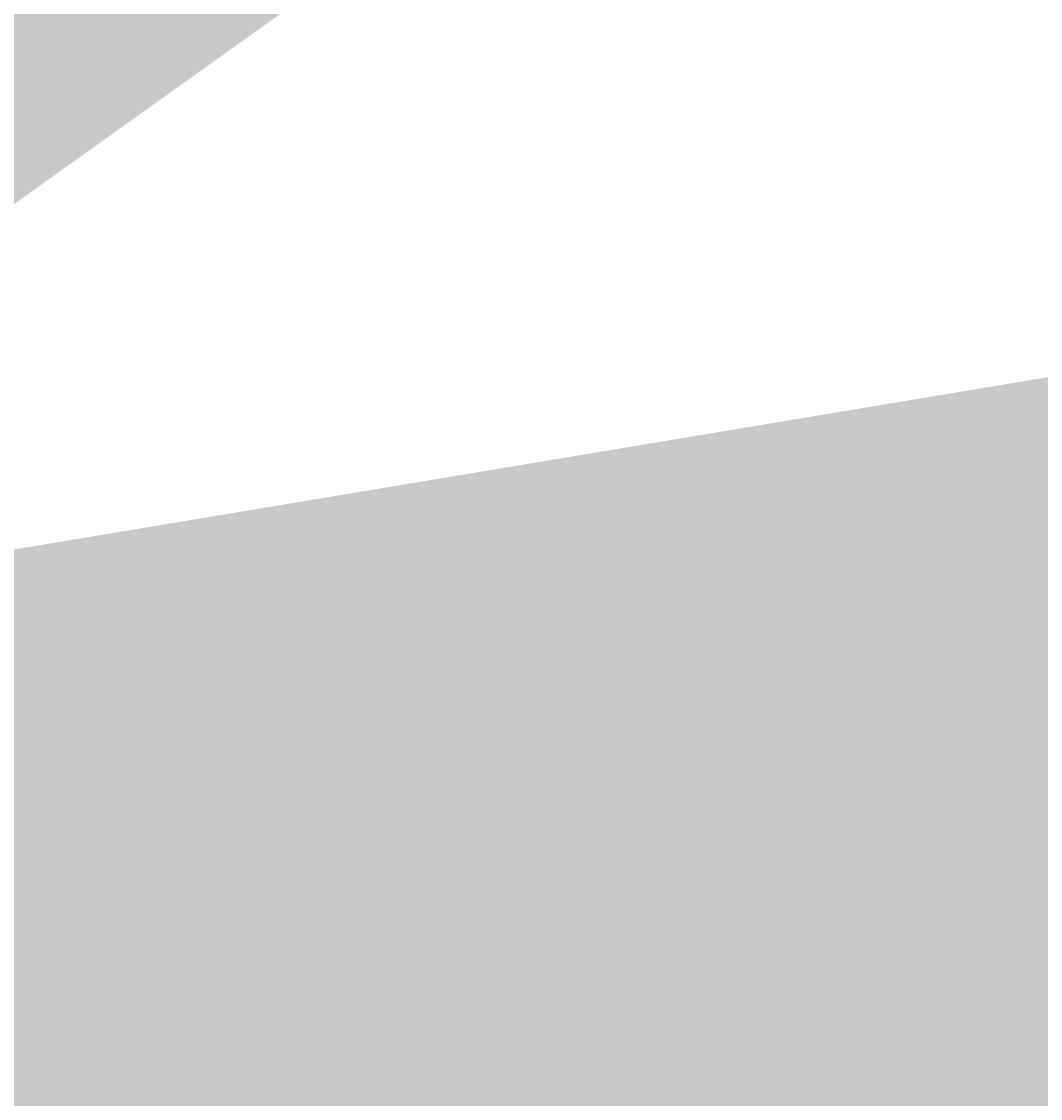
# Model space of a CAD drawing. Units: millimetres. Extents: x -22994 to 29398, y -19990 to 20176.
# Tile 129 of 135: x 1004 to 2052, y -212 to 895. Entities that reach past the tile are written whole.
import ezdxf

# ---------------------------------------------------------------- set-up
doc = ezdxf.new("R2010")
doc.units = ezdxf.units.MM
doc.header["$MEASUREMENT"] = 0
doc.layers.add('M-DIMS', color=2, linetype='Continuous', lineweight=18)
doc.styles.get("Standard").update_dxf_attribs({"font": 'arial.ttf'})
doc.dimstyles.get("Standard").update_dxf_attribs({"dimtxt": 0.18, "dimasz": 10000, "dimexe": 0.18, "dimexo": 0.0625, "dimgap": 0.09, "dimtad": 0, "dimtih": 1, "dimtoh": 1, "dimdec": 0, "dimzin": 0, "dimdsep": 46, "dimtxsty": 'Standard', "dimcen": 0.09, "dimadec": 0, "dimazin": 0, "dimtfac": 1, "dimtdec": 0, "dimtofl": 0, "dimtmove": 0, "dimatfit": 3, "dimfxl": 1, "dimtolj": 1, "dimtzin": 0, "dimlwd": 30, "dimarcsym": 0})

# ---------------------------------------------------------------- blocks, each defined once
blk = doc.blocks.new('*D2')
at = {"layer": 'Defpoints', "color": 0, "transparency": 16777216}
for p in [(6.7, 10.3), (290.9, 10.3), (290.9, -5.1)]:
    blk.add_point(p, dxfattribs=at)
at = {"layer": 'M-DIMS', "color": 0, "lineweight": -2, "transparency": 16777216}
for p, q in [((6.7, 10.2), (6.7, -5.3)), ((290.9, 10.2), (290.9, -5.3))]:
    blk.add_line(p, q, dxfattribs=at)
at = {"layer": 'M-DIMS', "color": 0, "lineweight": 30, "transparency": 16777216}
for p, q in [((-9993.3, -5.1), (-19993.3, -5.1)), ((10290.9, -5.1), (20290.9, -5.1))]:
    blk.add_line(p, q, dxfattribs=at)
at = {"layer": 'M-DIMS', "color": 0, "transparency": 16777216}
for points in [[(-9993.3, 1661.6), (-9993.3, -1671.7), (6.7, -5.1)], [(10290.9, 1661.6), (10290.9, -1671.7), (290.9, -5.1)]]:
    blk.add_solid(points, dxfattribs=at)
at = {"layer": 'M-DIMS', "color": 0, "transparency": 16777216, "insert": (148.8, -5.1), "char_height": 0.18, "attachment_point": 5}
blk.add_mtext('\\A1;284.2', dxfattribs=at)
blk = doc.blocks.new('*D3')
at = {"layer": 'Defpoints', "color": 0, "transparency": 16777216}
for p in [(110.3, 204.2), (110.3, 176.4), (95.8, 128)]:
    blk.add_point(p, dxfattribs=at)
at = {"layer": 'M-DIMS', "color": 0, "lineweight": 30, "transparency": 16777216}
for p, q in [((-9904.2, 204.2), (-19904.2, 204.2)), ((10110.3, 204.2), (20110.3, 204.2))]:
    blk.add_line(p, q, dxfattribs=at)
at = {"layer": 'M-DIMS', "color": 0, "lineweight": -2, "transparency": 16777216}
for p, q in [((95.8, 128), (95.8, 204.3)), ((110.3, 176.4), (110.3, 204.3))]:
    blk.add_line(p, q, dxfattribs=at)
at = {"layer": 'M-DIMS', "color": 0, "transparency": 16777216}
for points in [[(-9904.2, 1870.8), (-9904.2, -1462.5), (95.8, 204.2)], [(10110.3, 1870.8), (10110.3, -1462.5), (110.3, 204.2)]]:
    blk.add_solid(points, dxfattribs=at)
at = {"layer": 'M-DIMS', "color": 0, "transparency": 16777216, "insert": (103, 204.2), "char_height": 0.18, "attachment_point": 5}
blk.add_mtext('\\A1;14.432', dxfattribs=at)
blk = doc.blocks.new('*D4')
at = {"layer": 'Defpoints', "color": 0, "transparency": 16777216}
for p in [(116.3, 204.2), (110.3, 176.4), (116.3, 176.4)]:
    blk.add_point(p, dxfattribs=at)
at = {"layer": 'M-DIMS', "color": 0, "lineweight": 30, "transparency": 16777216}
for p, q in [((-9889.7, 204.2), (-19889.7, 204.2)), ((10116.3, 204.2), (20116.3, 204.2))]:
    blk.add_line(p, q, dxfattribs=at)
at = {"layer": 'M-DIMS', "color": 0, "lineweight": -2, "transparency": 16777216}
for p, q in [((110.3, 176.4), (110.3, 204.3)), ((116.3, 176.4), (116.3, 204.3))]:
    blk.add_line(p, q, dxfattribs=at)
at = {"layer": 'M-DIMS', "color": 0, "transparency": 16777216}
for points in [[(-9889.7, 1870.8), (-9889.7, -1462.5), (110.3, 204.2)], [(10116.3, 1870.8), (10116.3, -1462.5), (116.3, 204.2)]]:
    blk.add_solid(points, dxfattribs=at)
at = {"layer": 'M-DIMS', "color": 0, "transparency": 16777216, "insert": (113.3, 204.2), "char_height": 0.18, "attachment_point": 5}
blk.add_mtext('\\A1;6', dxfattribs=at)
blk = doc.blocks.new('*D5')
at = {"layer": 'Defpoints', "color": 0, "transparency": 16777216}
for p in [(181.3, 204.2), (116.3, 176.4), (181.3, 176.4)]:
    blk.add_point(p, dxfattribs=at)
at = {"layer": 'M-DIMS', "color": 0, "lineweight": 30, "transparency": 16777216}
for p, q in [((-9883.7, 204.2), (-19883.7, 204.2)), ((10181.3, 204.2), (20181.3, 204.2))]:
    blk.add_line(p, q, dxfattribs=at)
at = {"layer": 'M-DIMS', "color": 0, "lineweight": -2, "transparency": 16777216}
for p, q in [((116.3, 176.4), (116.3, 204.3)), ((181.3, 176.4), (181.3, 204.3))]:
    blk.add_line(p, q, dxfattribs=at)
at = {"layer": 'M-DIMS', "color": 0, "transparency": 16777216}
for points in [[(-9883.7, 1870.8), (-9883.7, -1462.5), (116.3, 204.2)], [(10181.3, 1870.8), (10181.3, -1462.5), (181.3, 204.2)]]:
    blk.add_solid(points, dxfattribs=at)
at = {"layer": 'M-DIMS', "color": 0, "transparency": 16777216, "insert": (148.8, 204.2), "char_height": 0.18, "attachment_point": 5}
blk.add_mtext('\\A1;65', dxfattribs=at)
blk = doc.blocks.new('*D6')
at = {"layer": 'Defpoints', "color": 0, "transparency": 16777216}
for p in [(187.3, 204.2), (181.3, 176.4), (187.3, 176.4)]:
    blk.add_point(p, dxfattribs=at)
at = {"layer": 'M-DIMS', "color": 0, "lineweight": 30, "transparency": 16777216}
for p, q in [((-9818.7, 204.2), (-19818.7, 204.2)), ((10187.3, 204.2), (20187.3, 204.2))]:
    blk.add_line(p, q, dxfattribs=at)
at = {"layer": 'M-DIMS', "color": 0, "lineweight": -2, "transparency": 16777216}
for p, q in [((181.3, 176.4), (181.3, 204.3)), ((187.3, 176.4), (187.3, 204.3))]:
    blk.add_line(p, q, dxfattribs=at)
at = {"layer": 'M-DIMS', "color": 0, "transparency": 16777216}
for points in [[(-9818.7, 1870.8), (-9818.7, -1462.5), (181.3, 204.2)], [(10187.3, 1870.8), (10187.3, -1462.5), (187.3, 204.2)]]:
    blk.add_solid(points, dxfattribs=at)
at = {"layer": 'M-DIMS', "color": 0, "transparency": 16777216, "insert": (184.3, 204.2), "char_height": 0.18, "attachment_point": 5}
blk.add_mtext('\\A1;6', dxfattribs=at)
blk = doc.blocks.new('*D7')
at = {"layer": 'Defpoints', "color": 0, "transparency": 16777216}
for p in [(201.7, 204.2), (187.3, 176.4), (201.7, 128)]:
    blk.add_point(p, dxfattribs=at)
at = {"layer": 'M-DIMS', "color": 0, "lineweight": 30, "transparency": 16777216}
for p, q in [((-9812.7, 204.2), (-19812.7, 204.2)), ((10201.7, 204.2), (20201.7, 204.2))]:
    blk.add_line(p, q, dxfattribs=at)
at = {"layer": 'M-DIMS', "color": 0, "lineweight": -2, "transparency": 16777216}
for p, q in [((187.3, 176.4), (187.3, 204.3)), ((201.7, 128), (201.7, 204.3))]:
    blk.add_line(p, q, dxfattribs=at)
at = {"layer": 'M-DIMS', "color": 0, "transparency": 16777216}
for points in [[(-9812.7, 1870.8), (-9812.7, -1462.5), (187.3, 204.2)], [(10201.7, 1870.8), (10201.7, -1462.5), (201.7, 204.2)]]:
    blk.add_solid(points, dxfattribs=at)
at = {"layer": 'M-DIMS', "color": 0, "transparency": 16777216, "insert": (194.5, 204.2), "char_height": 0.18, "attachment_point": 5}
blk.add_mtext('\\A1;14.432', dxfattribs=at)
blk = doc.blocks.new('*D8')
at = {"layer": 'Defpoints', "color": 0, "transparency": 16777216}
for p in [(227.6, 204.2), (227.6, 146.7), (201.7, 128)]:
    blk.add_point(p, dxfattribs=at)
at = {"layer": 'M-DIMS', "color": 0, "lineweight": 30, "transparency": 16777216}
for p, q in [((-9798.3, 204.2), (-19798.3, 204.2)), ((10227.6, 204.2), (20227.6, 204.2))]:
    blk.add_line(p, q, dxfattribs=at)
at = {"layer": 'M-DIMS', "color": 0, "lineweight": -2, "transparency": 16777216}
for p, q in [((201.7, 128), (201.7, 204.3)), ((227.6, 146.8), (227.6, 204.3))]:
    blk.add_line(p, q, dxfattribs=at)
at = {"layer": 'M-DIMS', "color": 0, "transparency": 16777216}
for points in [[(-9798.3, 1870.8), (-9798.3, -1462.5), (201.7, 204.2)], [(10227.6, 1870.8), (10227.6, -1462.5), (227.6, 204.2)]]:
    blk.add_solid(points, dxfattribs=at)
at = {"layer": 'M-DIMS', "color": 0, "transparency": 16777216, "insert": (214.7, 204.2), "char_height": 0.18, "attachment_point": 5}
blk.add_mtext('\\A1;25.95', dxfattribs=at)
blk = doc.blocks.new('*D9')
at = {"layer": 'Defpoints', "color": 0, "transparency": 16777216}
for p in [(187.3, 176.4), (306.2, 176.4), (290.9, 10.3)]:
    blk.add_point(p, dxfattribs=at)
at = {"layer": 'M-DIMS', "color": 0, "lineweight": 30, "transparency": 16777216}
for p, q in [((306.2, 10176.4), (306.2, 20176.4)), ((306.2, -9989.7), (306.2, -19989.7))]:
    blk.add_line(p, q, dxfattribs=at)
at = {"layer": 'M-DIMS', "color": 0, "lineweight": -2, "transparency": 16777216}
for p, q in [((187.3, 176.4), (306.4, 176.4)), ((290.9, 10.3), (306.4, 10.3))]:
    blk.add_line(p, q, dxfattribs=at)
at = {"layer": 'M-DIMS', "color": 0, "transparency": 16777216}
for points in [[(-1360.5, 10176.4), (1972.9, 10176.4), (306.2, 176.4)], [(-1360.5, -9989.7), (1972.9, -9989.7), (306.2, 10.3)]]:
    blk.add_solid(points, dxfattribs=at)
at = {"layer": 'M-DIMS', "color": 0, "transparency": 16777216, "insert": (306.2, 93.3), "char_height": 0.18, "attachment_point": 5}
blk.add_mtext('\\A1;166.1', dxfattribs=at)
blk = doc.blocks.new('*D10')
at = {"layer": 'Defpoints', "color": 0, "transparency": 16777216}
for p in [(125.6, 136.1), (133.3, 136.1), (133.3, -5.1)]:
    blk.add_point(p, dxfattribs=at)
at = {"layer": 'M-DIMS', "color": 0, "lineweight": -2, "transparency": 16777216}
for p, q in [((125.6, 136), (125.6, -5.3)), ((133.3, 136), (133.3, -5.3))]:
    blk.add_line(p, q, dxfattribs=at)
at = {"layer": 'M-DIMS', "color": 0, "lineweight": 30, "transparency": 16777216}
for p, q in [((-9874.4, -5.1), (-19874.4, -5.1)), ((10133.3, -5.1), (20133.3, -5.1))]:
    blk.add_line(p, q, dxfattribs=at)
at = {"layer": 'M-DIMS', "color": 0, "transparency": 16777216}
for points in [[(-9874.4, 1661.6), (-9874.4, -1671.7), (125.6, -5.1)], [(10133.3, 1661.6), (10133.3, -1671.7), (133.3, -5.1)]]:
    blk.add_solid(points, dxfattribs=at)
at = {"layer": 'M-DIMS', "color": 0, "transparency": 16777216, "insert": (129.5, -5.1), "char_height": 0.18, "attachment_point": 5}
blk.add_mtext('\\A1;7.696', dxfattribs=at)
blk = doc.blocks.new('*D11')
at = {"layer": 'Defpoints', "color": 0, "transparency": 16777216}
for p in [(133.3, 136.1), (135.6, 136.1), (135.6, -5.1)]:
    blk.add_point(p, dxfattribs=at)
at = {"layer": 'M-DIMS', "color": 0, "lineweight": -2, "transparency": 16777216}
for p, q in [((133.3, 136), (133.3, -5.3)), ((135.6, 136), (135.6, -5.3))]:
    blk.add_line(p, q, dxfattribs=at)
at = {"layer": 'M-DIMS', "color": 0, "lineweight": 30, "transparency": 16777216}
for p, q in [((-9866.7, -5.1), (-19866.7, -5.1)), ((10135.6, -5.1), (20135.6, -5.1))]:
    blk.add_line(p, q, dxfattribs=at)
at = {"layer": 'M-DIMS', "color": 0, "transparency": 16777216}
for points in [[(-9866.7, 1661.6), (-9866.7, -1671.7), (133.3, -5.1)], [(10135.6, 1661.6), (10135.6, -1671.7), (135.6, -5.1)]]:
    blk.add_solid(points, dxfattribs=at)
at = {"layer": 'M-DIMS', "color": 0, "transparency": 16777216, "insert": (134.5, -5.1), "char_height": 0.18, "attachment_point": 5}
blk.add_mtext('\\A1;2.304', dxfattribs=at)
blk = doc.blocks.new('*D12')
at = {"layer": 'Defpoints', "color": 0, "transparency": 16777216}
for p in [(135.6, 136.1), (145.6, 136.1), (145.6, -5.1)]:
    blk.add_point(p, dxfattribs=at)
at = {"layer": 'M-DIMS', "color": 0, "lineweight": -2, "transparency": 16777216}
for p, q in [((135.6, 136), (135.6, -5.3)), ((145.6, 136), (145.6, -5.3))]:
    blk.add_line(p, q, dxfattribs=at)
at = {"layer": 'M-DIMS', "color": 0, "lineweight": 30, "transparency": 16777216}
for p, q in [((-9864.4, -5.1), (-19864.4, -5.1)), ((10145.6, -5.1), (20145.6, -5.1))]:
    blk.add_line(p, q, dxfattribs=at)
at = {"layer": 'M-DIMS', "color": 0, "transparency": 16777216}
for points in [[(-9864.4, 1661.6), (-9864.4, -1671.7), (135.6, -5.1)], [(10145.6, 1661.6), (10145.6, -1671.7), (145.6, -5.1)]]:
    blk.add_solid(points, dxfattribs=at)
at = {"layer": 'M-DIMS', "color": 0, "transparency": 16777216, "insert": (140.6, -5.1), "char_height": 0.18, "attachment_point": 5}
blk.add_mtext('\\A1;10', dxfattribs=at)
blk = doc.blocks.new('*D13')
at = {"layer": 'Defpoints', "color": 0, "transparency": 16777216}
for p in [(145.6, 136.1), (155.6, 136.1), (155.6, -5.1)]:
    blk.add_point(p, dxfattribs=at)
at = {"layer": 'M-DIMS', "color": 0, "lineweight": -2, "transparency": 16777216}
for p, q in [((145.6, 136), (145.6, -5.3)), ((155.6, 136), (155.6, -5.3))]:
    blk.add_line(p, q, dxfattribs=at)
at = {"layer": 'M-DIMS', "color": 0, "lineweight": 30, "transparency": 16777216}
for p, q in [((-9854.4, -5.1), (-19854.4, -5.1)), ((10155.6, -5.1), (20155.6, -5.1))]:
    blk.add_line(p, q, dxfattribs=at)
at = {"layer": 'M-DIMS', "color": 0, "transparency": 16777216}
for points in [[(-9854.4, 1661.6), (-9854.4, -1671.7), (145.6, -5.1)], [(10155.6, 1661.6), (10155.6, -1671.7), (155.6, -5.1)]]:
    blk.add_solid(points, dxfattribs=at)
at = {"layer": 'M-DIMS', "color": 0, "transparency": 16777216, "insert": (150.6, -5.1), "char_height": 0.18, "attachment_point": 5}
blk.add_mtext('\\A1;10', dxfattribs=at)
blk = doc.blocks.new('*D14')
at = {"layer": 'Defpoints', "color": 0, "transparency": 16777216}
for p in [(155.6, 136.1), (165.6, 136.1), (165.6, -5.1)]:
    blk.add_point(p, dxfattribs=at)
at = {"layer": 'M-DIMS', "color": 0, "lineweight": -2, "transparency": 16777216}
for p, q in [((155.6, 136), (155.6, -5.3)), ((165.6, 136), (165.6, -5.3))]:
    blk.add_line(p, q, dxfattribs=at)
at = {"layer": 'M-DIMS', "color": 0, "lineweight": 30, "transparency": 16777216}
for p, q in [((-9844.4, -5.1), (-19844.4, -5.1)), ((10165.6, -5.1), (20165.6, -5.1))]:
    blk.add_line(p, q, dxfattribs=at)
at = {"layer": 'M-DIMS', "color": 0, "transparency": 16777216}
for points in [[(-9844.4, 1661.6), (-9844.4, -1671.7), (155.6, -5.1)], [(10165.6, 1661.6), (10165.6, -1671.7), (165.6, -5.1)]]:
    blk.add_solid(points, dxfattribs=at)
at = {"layer": 'M-DIMS', "color": 0, "transparency": 16777216, "insert": (160.6, -5.1), "char_height": 0.18, "attachment_point": 5}
blk.add_mtext('\\A1;10', dxfattribs=at)
blk = doc.blocks.new('*D15')
at = {"layer": 'Defpoints', "color": 0, "transparency": 16777216}
for p in [(173.3, 154.8), (173.3, 136.1), (306.2, 136.1)]:
    blk.add_point(p, dxfattribs=at)
at = {"layer": 'M-DIMS', "color": 0, "lineweight": 30, "transparency": 16777216}
for p, q in [((306.2, 10154.8), (306.2, 20154.8)), ((306.2, -9863.9), (306.2, -19863.9))]:
    blk.add_line(p, q, dxfattribs=at)
at = {"layer": 'M-DIMS', "color": 0, "lineweight": -2, "transparency": 16777216}
for p, q in [((173.4, 154.8), (306.4, 154.8)), ((173.4, 136.1), (306.4, 136.1))]:
    blk.add_line(p, q, dxfattribs=at)
at = {"layer": 'M-DIMS', "color": 0, "transparency": 16777216}
for points in [[(-1360.5, 10154.8), (1972.9, 10154.8), (306.2, 154.8)], [(-1360.5, -9863.9), (1972.9, -9863.9), (306.2, 136.1)]]:
    blk.add_solid(points, dxfattribs=at)
at = {"layer": 'M-DIMS', "color": 0, "transparency": 16777216, "insert": (306.2, 145.4), "char_height": 0.18, "attachment_point": 5}
blk.add_mtext('\\A1;18.717', dxfattribs=at)
blk = doc.blocks.new('*D16')
at = {"layer": 'Defpoints', "color": 0, "transparency": 16777216}
for p in [(120.2, 204.2), (110.5, 48), (120.2, 48)]:
    blk.add_point(p, dxfattribs=at)
at = {"layer": 'M-DIMS', "color": 0, "lineweight": 30, "transparency": 16777216}
for p, q in [((-9889.5, 204.2), (-19889.5, 204.2)), ((10120.2, 204.2), (20120.2, 204.2))]:
    blk.add_line(p, q, dxfattribs=at)
at = {"layer": 'M-DIMS', "color": 0, "lineweight": -2, "transparency": 16777216}
for p, q in [((110.5, 48.1), (110.5, 204.3)), ((120.2, 48.1), (120.2, 204.3))]:
    blk.add_line(p, q, dxfattribs=at)
at = {"layer": 'M-DIMS', "color": 0, "transparency": 16777216}
for points in [[(-9889.5, 1870.8), (-9889.5, -1462.5), (110.5, 204.2)], [(10120.2, 1870.8), (10120.2, -1462.5), (120.2, 204.2)]]:
    blk.add_solid(points, dxfattribs=at)
at = {"layer": 'M-DIMS', "color": 0, "transparency": 16777216, "insert": (115.3, 204.2), "char_height": 0.18, "attachment_point": 5}
blk.add_mtext('\\A1;9.704', dxfattribs=at)
blk = doc.blocks.new('*D17')
at = {"layer": 'Defpoints', "color": 0, "transparency": 16777216}
for p in [(126.2, 204.2), (120.2, 48), (126.2, 48)]:
    blk.add_point(p, dxfattribs=at)
at = {"layer": 'M-DIMS', "color": 0, "lineweight": 30, "transparency": 16777216}
for p, q in [((-9879.8, 204.2), (-19879.8, 204.2)), ((10126.2, 204.2), (20126.2, 204.2))]:
    blk.add_line(p, q, dxfattribs=at)
at = {"layer": 'M-DIMS', "color": 0, "lineweight": -2, "transparency": 16777216}
for p, q in [((120.2, 48.1), (120.2, 204.3)), ((126.2, 48.1), (126.2, 204.3))]:
    blk.add_line(p, q, dxfattribs=at)
at = {"layer": 'M-DIMS', "color": 0, "transparency": 16777216}
for points in [[(-9879.8, 1870.8), (-9879.8, -1462.5), (120.2, 204.2)], [(10126.2, 1870.8), (10126.2, -1462.5), (126.2, 204.2)]]:
    blk.add_solid(points, dxfattribs=at)
at = {"layer": 'M-DIMS', "color": 0, "transparency": 16777216, "insert": (123.2, 204.2), "char_height": 0.18, "attachment_point": 5}
blk.add_mtext('\\A1;6', dxfattribs=at)
blk = doc.blocks.new('*D18')
at = {"layer": 'Defpoints', "color": 0, "transparency": 16777216}
for p in [(132.2, 204.2), (126.2, 48), (132.2, 48)]:
    blk.add_point(p, dxfattribs=at)
at = {"layer": 'M-DIMS', "color": 0, "lineweight": 30, "transparency": 16777216}
for p, q in [((-9873.8, 204.2), (-19873.8, 204.2)), ((10132.2, 204.2), (20132.2, 204.2))]:
    blk.add_line(p, q, dxfattribs=at)
at = {"layer": 'M-DIMS', "color": 0, "lineweight": -2, "transparency": 16777216}
for p, q in [((126.2, 48.1), (126.2, 204.3)), ((132.2, 48.1), (132.2, 204.3))]:
    blk.add_line(p, q, dxfattribs=at)
at = {"layer": 'M-DIMS', "color": 0, "transparency": 16777216}
for points in [[(-9873.8, 1870.8), (-9873.8, -1462.5), (126.2, 204.2)], [(10132.2, 1870.8), (10132.2, -1462.5), (132.2, 204.2)]]:
    blk.add_solid(points, dxfattribs=at)
at = {"layer": 'M-DIMS', "color": 0, "transparency": 16777216, "insert": (129.2, 204.2), "char_height": 0.18, "attachment_point": 5}
blk.add_mtext('\\A1;6', dxfattribs=at)
blk = doc.blocks.new('*D19')
at = {"layer": 'Defpoints', "color": 0, "transparency": 16777216}
for p in [(138.2, 204.2), (132.2, 48), (138.2, 48)]:
    blk.add_point(p, dxfattribs=at)
at = {"layer": 'M-DIMS', "color": 0, "lineweight": 30, "transparency": 16777216}
for p, q in [((-9867.8, 204.2), (-19867.8, 204.2)), ((10138.2, 204.2), (20138.2, 204.2))]:
    blk.add_line(p, q, dxfattribs=at)
at = {"layer": 'M-DIMS', "color": 0, "lineweight": -2, "transparency": 16777216}
for p, q in [((132.2, 48.1), (132.2, 204.3)), ((138.2, 48.1), (138.2, 204.3))]:
    blk.add_line(p, q, dxfattribs=at)
at = {"layer": 'M-DIMS', "color": 0, "transparency": 16777216}
for points in [[(-9867.8, 1870.8), (-9867.8, -1462.5), (132.2, 204.2)], [(10138.2, 1870.8), (10138.2, -1462.5), (138.2, 204.2)]]:
    blk.add_solid(points, dxfattribs=at)
at = {"layer": 'M-DIMS', "color": 0, "transparency": 16777216, "insert": (135.2, 204.2), "char_height": 0.18, "attachment_point": 5}
blk.add_mtext('\\A1;6', dxfattribs=at)
blk = doc.blocks.new('*D20')
at = {"layer": 'Defpoints', "color": 0, "transparency": 16777216}
for p in [(144.2, 204.2), (138.2, 48), (144.2, 48)]:
    blk.add_point(p, dxfattribs=at)
at = {"layer": 'M-DIMS', "color": 0, "lineweight": 30, "transparency": 16777216}
for p, q in [((-9861.8, 204.2), (-19861.8, 204.2)), ((10144.2, 204.2), (20144.2, 204.2))]:
    blk.add_line(p, q, dxfattribs=at)
at = {"layer": 'M-DIMS', "color": 0, "lineweight": -2, "transparency": 16777216}
for p, q in [((138.2, 48.1), (138.2, 204.3)), ((144.2, 48.1), (144.2, 204.3))]:
    blk.add_line(p, q, dxfattribs=at)
at = {"layer": 'M-DIMS', "color": 0, "transparency": 16777216}
for points in [[(-9861.8, 1870.8), (-9861.8, -1462.5), (138.2, 204.2)], [(10144.2, 1870.8), (10144.2, -1462.5), (144.2, 204.2)]]:
    blk.add_solid(points, dxfattribs=at)
at = {"layer": 'M-DIMS', "color": 0, "transparency": 16777216, "insert": (141.2, 204.2), "char_height": 0.18, "attachment_point": 5}
blk.add_mtext('\\A1;6', dxfattribs=at)
blk = doc.blocks.new('*D21')
at = {"layer": 'Defpoints', "color": 0, "transparency": 16777216}
for p in [(149.1, 204.2), (144.2, 48), (149.1, 48)]:
    blk.add_point(p, dxfattribs=at)
at = {"layer": 'M-DIMS', "color": 0, "lineweight": 30, "transparency": 16777216}
for p, q in [((-9855.8, 204.2), (-19855.8, 204.2)), ((10149.1, 204.2), (20149.1, 204.2))]:
    blk.add_line(p, q, dxfattribs=at)
at = {"layer": 'M-DIMS', "color": 0, "lineweight": -2, "transparency": 16777216}
for p, q in [((144.2, 48.1), (144.2, 204.3)), ((149.1, 48.1), (149.1, 204.3))]:
    blk.add_line(p, q, dxfattribs=at)
at = {"layer": 'M-DIMS', "color": 0, "transparency": 16777216}
for points in [[(-9855.8, 1870.8), (-9855.8, -1462.5), (144.2, 204.2)], [(10149.1, 1870.8), (10149.1, -1462.5), (149.1, 204.2)]]:
    blk.add_solid(points, dxfattribs=at)
at = {"layer": 'M-DIMS', "color": 0, "transparency": 16777216, "insert": (146.6, 204.2), "char_height": 0.18, "attachment_point": 5}
blk.add_mtext('\\A1;4.945', dxfattribs=at)
blk = doc.blocks.new('*D22')
at = {"layer": 'Defpoints', "color": 0, "transparency": 16777216}
for p in [(149.1, 31), (155.1, 31), (155.1, -5.1)]:
    blk.add_point(p, dxfattribs=at)
at = {"layer": 'M-DIMS', "color": 0, "lineweight": -2, "transparency": 16777216}
for p, q in [((149.1, 30.9), (149.1, -5.3)), ((155.1, 30.9), (155.1, -5.3))]:
    blk.add_line(p, q, dxfattribs=at)
at = {"layer": 'M-DIMS', "color": 0, "lineweight": 30, "transparency": 16777216}
for p, q in [((-9850.9, -5.1), (-19850.9, -5.1)), ((10155.1, -5.1), (20155.1, -5.1))]:
    blk.add_line(p, q, dxfattribs=at)
at = {"layer": 'M-DIMS', "color": 0, "transparency": 16777216}
for points in [[(-9850.9, 1661.6), (-9850.9, -1671.7), (149.1, -5.1)], [(10155.1, 1661.6), (10155.1, -1671.7), (155.1, -5.1)]]:
    blk.add_solid(points, dxfattribs=at)
at = {"layer": 'M-DIMS', "color": 0, "transparency": 16777216, "insert": (152.1, -5.1), "char_height": 0.18, "attachment_point": 5}
blk.add_mtext('\\A1;6', dxfattribs=at)
blk = doc.blocks.new('*D23')
at = {"layer": 'Defpoints', "color": 0, "transparency": 16777216}
for p in [(155.1, 31), (161.1, 31), (161.1, -5.1)]:
    blk.add_point(p, dxfattribs=at)
at = {"layer": 'M-DIMS', "color": 0, "lineweight": -2, "transparency": 16777216}
for p, q in [((155.1, 30.9), (155.1, -5.3)), ((161.1, 30.9), (161.1, -5.3))]:
    blk.add_line(p, q, dxfattribs=at)
at = {"layer": 'M-DIMS', "color": 0, "lineweight": 30, "transparency": 16777216}
for p, q in [((-9844.9, -5.1), (-19844.9, -5.1)), ((10161.1, -5.1), (20161.1, -5.1))]:
    blk.add_line(p, q, dxfattribs=at)
at = {"layer": 'M-DIMS', "color": 0, "transparency": 16777216}
for points in [[(-9844.9, 1661.6), (-9844.9, -1671.7), (155.1, -5.1)], [(10161.1, 1661.6), (10161.1, -1671.7), (161.1, -5.1)]]:
    blk.add_solid(points, dxfattribs=at)
at = {"layer": 'M-DIMS', "color": 0, "transparency": 16777216, "insert": (158.1, -5.1), "char_height": 0.18, "attachment_point": 5}
blk.add_mtext('\\A1;6', dxfattribs=at)
blk = doc.blocks.new('*D24')
at = {"layer": 'Defpoints', "color": 0, "transparency": 16777216}
for p in [(161.1, 31), (166.4, 31), (166.4, -5.1)]:
    blk.add_point(p, dxfattribs=at)
at = {"layer": 'M-DIMS', "color": 0, "lineweight": -2, "transparency": 16777216}
for p, q in [((161.1, 30.9), (161.1, -5.3)), ((166.4, 30.9), (166.4, -5.3))]:
    blk.add_line(p, q, dxfattribs=at)
at = {"layer": 'M-DIMS', "color": 0, "lineweight": 30, "transparency": 16777216}
for p, q in [((-9838.9, -5.1), (-19838.9, -5.1)), ((10166.4, -5.1), (20166.4, -5.1))]:
    blk.add_line(p, q, dxfattribs=at)
at = {"layer": 'M-DIMS', "color": 0, "transparency": 16777216}
for points in [[(-9838.9, 1661.6), (-9838.9, -1671.7), (161.1, -5.1)], [(10166.4, 1661.6), (10166.4, -1671.7), (166.4, -5.1)]]:
    blk.add_solid(points, dxfattribs=at)
at = {"layer": 'M-DIMS', "color": 0, "transparency": 16777216, "insert": (163.8, -5.1), "char_height": 0.18, "attachment_point": 5}
blk.add_mtext('\\A1;5.323', dxfattribs=at)
blk = doc.blocks.new('*D25')
at = {"layer": 'Defpoints', "color": 0, "transparency": 16777216}
for p in [(166.4, 31), (172.4, 31), (172.4, -5.1)]:
    blk.add_point(p, dxfattribs=at)
at = {"layer": 'M-DIMS', "color": 0, "lineweight": -2, "transparency": 16777216}
for p, q in [((166.4, 30.9), (166.4, -5.3)), ((172.4, 30.9), (172.4, -5.3))]:
    blk.add_line(p, q, dxfattribs=at)
at = {"layer": 'M-DIMS', "color": 0, "lineweight": 30, "transparency": 16777216}
for p, q in [((-9833.6, -5.1), (-19833.6, -5.1)), ((10172.4, -5.1), (20172.4, -5.1))]:
    blk.add_line(p, q, dxfattribs=at)
at = {"layer": 'M-DIMS', "color": 0, "transparency": 16777216}
for points in [[(-9833.6, 1661.6), (-9833.6, -1671.7), (166.4, -5.1)], [(10172.4, 1661.6), (10172.4, -1671.7), (172.4, -5.1)]]:
    blk.add_solid(points, dxfattribs=at)
at = {"layer": 'M-DIMS', "color": 0, "transparency": 16777216, "insert": (169.4, -5.1), "char_height": 0.18, "attachment_point": 5}
blk.add_mtext('\\A1;6', dxfattribs=at)
blk = doc.blocks.new('*D26')
at = {"layer": 'Defpoints', "color": 0, "transparency": 16777216}
for p in [(172.4, 31), (178.4, 31), (178.4, -5.1)]:
    blk.add_point(p, dxfattribs=at)
at = {"layer": 'M-DIMS', "color": 0, "lineweight": -2, "transparency": 16777216}
for p, q in [((172.4, 30.9), (172.4, -5.3)), ((178.4, 30.9), (178.4, -5.3))]:
    blk.add_line(p, q, dxfattribs=at)
at = {"layer": 'M-DIMS', "color": 0, "lineweight": 30, "transparency": 16777216}
for p, q in [((-9827.6, -5.1), (-19827.6, -5.1)), ((10178.4, -5.1), (20178.4, -5.1))]:
    blk.add_line(p, q, dxfattribs=at)
at = {"layer": 'M-DIMS', "color": 0, "transparency": 16777216}
for points in [[(-9827.6, 1661.6), (-9827.6, -1671.7), (172.4, -5.1)], [(10178.4, 1661.6), (10178.4, -1671.7), (178.4, -5.1)]]:
    blk.add_solid(points, dxfattribs=at)
at = {"layer": 'M-DIMS', "color": 0, "transparency": 16777216, "insert": (175.4, -5.1), "char_height": 0.18, "attachment_point": 5}
blk.add_mtext('\\A1;6', dxfattribs=at)
blk = doc.blocks.new('*D27')
at = {"layer": 'Defpoints', "color": 0, "transparency": 16777216}
for p in [(178.4, 31), (188.1, 31), (188.1, -5.1)]:
    blk.add_point(p, dxfattribs=at)
at = {"layer": 'M-DIMS', "color": 0, "lineweight": -2, "transparency": 16777216}
for p, q in [((178.4, 30.9), (178.4, -5.3)), ((188.1, 30.9), (188.1, -5.3))]:
    blk.add_line(p, q, dxfattribs=at)
at = {"layer": 'M-DIMS', "color": 0, "lineweight": 30, "transparency": 16777216}
for p, q in [((-9821.6, -5.1), (-19821.6, -5.1)), ((10188.1, -5.1), (20188.1, -5.1))]:
    blk.add_line(p, q, dxfattribs=at)
at = {"layer": 'M-DIMS', "color": 0, "transparency": 16777216}
for points in [[(-9821.6, 1661.6), (-9821.6, -1671.7), (178.4, -5.1)], [(10188.1, 1661.6), (10188.1, -1671.7), (188.1, -5.1)]]:
    blk.add_solid(points, dxfattribs=at)
at = {"layer": 'M-DIMS', "color": 0, "transparency": 16777216, "insert": (183.3, -5.1), "char_height": 0.18, "attachment_point": 5}
blk.add_mtext('\\A1;9.679', dxfattribs=at)
blk = doc.blocks.new('*D28')
at = {"layer": 'Defpoints', "color": 0, "transparency": 16777216}
for p in [(188.1, 48), (306.2, 48), (188.1, 31)]:
    blk.add_point(p, dxfattribs=at)
at = {"layer": 'M-DIMS', "color": 0, "lineweight": 30, "transparency": 16777216}
for p, q in [((306.2, 10048), (306.2, 20048)), ((306.2, -9969), (306.2, -19969))]:
    blk.add_line(p, q, dxfattribs=at)
at = {"layer": 'M-DIMS', "color": 0, "lineweight": -2, "transparency": 16777216}
for p, q in [((188.2, 48), (306.4, 48)), ((188.2, 31), (306.4, 31))]:
    blk.add_line(p, q, dxfattribs=at)
at = {"layer": 'M-DIMS', "color": 0, "transparency": 16777216}
for points in [[(-1360.5, 10048), (1972.9, 10048), (306.2, 48)], [(-1360.5, -9969), (1972.9, -9969), (306.2, 31)]]:
    blk.add_solid(points, dxfattribs=at)
at = {"layer": 'M-DIMS', "color": 0, "transparency": 16777216, "insert": (306.2, 39.5), "char_height": 0.18, "attachment_point": 5}
blk.add_mtext('\\A1;17.045', dxfattribs=at)
blk = doc.blocks.new('*D29')
at = {"layer": 'Defpoints', "color": 0, "transparency": 16777216}
for p in [(36.8, 80), (64, 80)]:
    blk.add_point(p, dxfattribs=at)
at = {"layer": 'M-DIMS', "color": 0, "lineweight": -2, "transparency": 16777216}
for p, q in [((50.3, 80), (50.5, 80)), ((50.4, 80), (50.4, 80.1))]:
    blk.add_line(p, q, dxfattribs=at)
at = {"layer": 'M-DIMS', "color": 0, "lineweight": 30, "transparency": 16777216}
blk.add_line((20064, 80), (10064, 80), dxfattribs=at)
at = {"layer": 'M-DIMS', "color": 0, "transparency": 16777216}
blk.add_solid([(10064, 1746.7), (10064, -1586.6), (64, 80)], dxfattribs=at)
at = {"layer": 'M-DIMS', "color": 0, "transparency": 16777216, "insert": (20064.5, 80), "char_height": 0.18, "attachment_point": 5}
blk.add_mtext('\\A1;∅27.23', dxfattribs=at)
blk = doc.blocks.new('*D30')
at = {"layer": 'Defpoints', "color": 0, "transparency": 16777216}
for p in [(216.3, 146.7), (239, 146.7)]:
    blk.add_point(p, dxfattribs=at)
at = {"layer": 'M-DIMS', "color": 0, "lineweight": -2, "transparency": 16777216}
for p, q in [((227.6, 146.6), (227.6, 146.8)), ((227.6, 146.7), (227.7, 146.7))]:
    blk.add_line(p, q, dxfattribs=at)
at = {"layer": 'M-DIMS', "color": 0, "lineweight": 30, "transparency": 16777216}
blk.add_line((20239, 147.5), (10239, 147.1), dxfattribs=at)
at = {"layer": 'M-DIMS', "color": 0, "transparency": 16777216}
blk.add_solid([(10238.9, 1813.8), (10239, -1519.6), (239, 146.7)], dxfattribs=at)
at = {"layer": 'M-DIMS', "color": 0, "transparency": 16777216, "insert": (20239.5, 147.5), "char_height": 0.18, "attachment_point": 5}
blk.add_mtext('\\A1;∅22.667', dxfattribs=at)
blk = doc.blocks.new('*D31')
at = {"layer": 'Defpoints', "color": 0, "transparency": 16777216}
for p in [(223.2, 146.7), (232.1, 146.7)]:
    blk.add_point(p, dxfattribs=at)
at = {"layer": 'M-DIMS', "color": 0, "lineweight": -2, "transparency": 16777216}
for p, q in [((227.6, 146.6), (227.6, 146.8)), ((227.6, 146.7), (227.7, 146.7))]:
    blk.add_line(p, q, dxfattribs=at)
at = {"layer": 'M-DIMS', "color": 0, "lineweight": 30, "transparency": 16777216}
blk.add_line((20232.1, 148.7), (10232.1, 147.7), dxfattribs=at)
at = {"layer": 'M-DIMS', "color": 0, "transparency": 16777216}
blk.add_solid([(10232, 1814.4), (10232.3, -1519), (232.1, 146.7)], dxfattribs=at)
at = {"layer": 'M-DIMS', "color": 0, "transparency": 16777216, "insert": (20232.6, 148.7), "char_height": 0.18, "attachment_point": 5}
blk.add_mtext('\\A1;∅8.969', dxfattribs=at)
blk = doc.blocks.new('*D33')
at = {"layer": 'Defpoints', "color": 0, "transparency": 16777216}
for p in [(229.6, 154.4), (233, 153.4)]:
    blk.add_point(p, dxfattribs=at)
at = {"layer": 'M-DIMS', "color": 0, "lineweight": -2, "transparency": 16777216}
for p, q in [((229.5, 154.4), (229.7, 154.4)), ((229.6, 154.3), (229.6, 154.5))]:
    blk.add_line(p, q, dxfattribs=at)
at = {"layer": 'M-DIMS', "color": 0, "lineweight": 30, "transparency": 16777216}
for p, q in [((19396.3, -5570.8), (9814.7, -2708.7)), ((29396.3, -5570.8), (19396.3, -5570.8))]:
    blk.add_line(p, q, dxfattribs=at)
at = {"layer": 'M-DIMS', "color": 0, "transparency": 16777216}
blk.add_solid([(10291.7, -1111.8), (9337.7, -4305.7), (233, 153.4)], dxfattribs=at)
at = {"layer": 'M-DIMS', "color": 0, "transparency": 16777216, "insert": (29397, -5570.8), "char_height": 0.18, "attachment_point": 5}
blk.add_mtext('\\A1;6X R3.586', dxfattribs=at)
blk = doc.blocks.new('*D34')
at = {"layer": 'Defpoints', "color": 0, "transparency": 16777216}
for p in [(178.6, 122.9), (176.8, 121.1)]:
    blk.add_point(p, dxfattribs=at)
at = {"layer": 'M-DIMS', "color": 0, "lineweight": 30, "transparency": 16777216}
for p, q in [((14322.4, 14263.3), (7250.5, 7193.1)), ((24322.4, 14263.3), (14322.4, 14263.3))]:
    blk.add_line(p, q, dxfattribs=at)
at = {"layer": 'M-DIMS', "color": 0, "lineweight": -2, "transparency": 16777216}
for p, q in [((176.7, 121.1), (176.9, 121.1)), ((176.8, 121), (176.8, 121.2))]:
    blk.add_line(p, q, dxfattribs=at)
at = {"layer": 'M-DIMS', "color": 0, "transparency": 16777216}
blk.add_solid([(6072.1, 8371.8), (8428.9, 6014.4), (178.6, 122.9)], dxfattribs=at)
at = {"layer": 'M-DIMS', "color": 0, "transparency": 16777216, "insert": (24323, 14263.3), "char_height": 0.18, "attachment_point": 5}
blk.add_mtext('\\A1;6X R2.5', dxfattribs=at)
blk = doc.blocks.new('*D36')
at = {"layer": 'Defpoints', "color": 0, "transparency": 16777216}
for p in [(46.4, 31.3), (46.4, 26.6)]:
    blk.add_point(p, dxfattribs=at)
at = {"layer": 'M-DIMS', "color": 0, "lineweight": 30, "transparency": 16777216}
for p, q in [((57.1, 20031.3), (51.8, 10031.3)), ((10057.1, 20031.3), (57.1, 20031.3))]:
    blk.add_line(p, q, dxfattribs=at)
at = {"layer": 'M-DIMS', "color": 0, "lineweight": -2, "transparency": 16777216}
for p, q in [((46.3, 28.9), (46.5, 28.9)), ((46.4, 28.9), (46.4, 29))]:
    blk.add_line(p, q, dxfattribs=at)
at = {"layer": 'M-DIMS', "color": 0, "transparency": 16777216}
blk.add_solid([(-1614.9, 10032.2), (1718.4, 10030.4), (46.4, 31.3)], dxfattribs=at)
at = {"layer": 'M-DIMS', "color": 0, "transparency": 16777216, "insert": (10057.6, 20031.3), "char_height": 0.18, "attachment_point": 5}
blk.add_mtext('\\A1;∅4.71', dxfattribs=at)
blk = doc.blocks.new('*D37')
at = {"layer": 'Defpoints', "color": 0, "transparency": 16777216}
for p in [(54.8, 118.6), (59.5, 118.6)]:
    blk.add_point(p, dxfattribs=at)
at = {"layer": 'M-DIMS', "color": 0, "lineweight": -2, "transparency": 16777216}
for p, q in [((57.1, 118.6), (57.3, 118.6)), ((57.2, 118.5), (57.2, 118.7))]:
    blk.add_line(p, q, dxfattribs=at)
at = {"layer": 'M-DIMS', "color": 0, "lineweight": 30, "transparency": 16777216}
blk.add_line((20059.5, 116.3), (10059.5, 117.4), dxfattribs=at)
at = {"layer": 'M-DIMS', "color": 0, "transparency": 16777216}
blk.add_solid([(10059.7, 1784.1), (10059.3, -1549.2), (59.5, 118.6)], dxfattribs=at)
at = {"layer": 'M-DIMS', "color": 0, "transparency": 16777216, "insert": (20060, 116.3), "char_height": 0.18, "attachment_point": 5}
blk.add_mtext('\\A1;∅4.659', dxfattribs=at)

msp = doc.modelspace()

# ---------------------------------------------------------------- dimensions: what is measured, and where the dimension line sits
at = {"layer": 'M-DIMS'}
for base, p1, p2, override, picture, middle in [((306.202, 176.3662), (290.852, 10.2713), (187.2647, 176.3662), {"dimdec": 1, "dimlfac": 1, "dimrnd": 0, "dimzin": 0, "dimdsep": 46, "dimlunit": 2}, '*D9', (306.202, 93.3187)), ((306.202, 136.0713), (173.3459, 154.788), (173.3459, 136.0713), {"dimdec": 3, "dimlfac": 1, "dimrnd": 0, "dimzin": 0, "dimdsep": 46, "dimlunit": 2}, '*D15', (306.202, 145.4297)), ((306.202, 48.0349), (188.1175, 30.9895), (188.1175, 48.0349), {"dimdec": 3, "dimlfac": 1, "dimrnd": 0, "dimzin": 0, "dimdsep": 46, "dimlunit": 2}, '*D28', (306.202, 39.5122))]:
    dim = msp.add_linear_dim(base=base, p1=p1, p2=p2, angle=90, dimstyle='Standard', override=override, dxfattribs=at)
    dim.commit()
    dim.dimension.update_dxf_attribs({"geometry": picture, "text_midpoint": middle})
for p1, p2, override, picture, middle in [((46.3875, 26.5934), (46.39, 31.3035), {"dimdec": 2, "dimlfac": 1, "dimrnd": 0, "dimzin": 0, "dimdsep": 46, "dimlunit": 2}, '*D36', (10057.5542, 20031.3006)), ((216.3148, 146.7291), (238.9821, 146.73), {"dimdec": 3, "dimlfac": 1, "dimrnd": 0, "dimzin": 0, "dimdsep": 46, "dimlunit": 2}, '*D30', (20238.9821, 147.4959)), ((223.1641, 146.7291), (232.1328, 146.73), {"dimdec": 3, "dimlfac": 1, "dimrnd": 0, "dimzin": 0, "dimdsep": 46, "dimlunit": 2}, '*D31', (20232.1327, 148.6656))]:
    dim = msp.add_diameter_dim_2p(p1=p1, p2=p2, dimstyle='Standard', override=override, dxfattribs=at)
    dim.commit()
    dim.dimension.update_dxf_attribs({"geometry": picture, "text_midpoint": middle, "dimtype": 163})
for center, mpoint, override, picture, middle in [((176.8123, 121.1277), (178.5802, 122.8952), {"dimdec": 1, "dimlfac": 1, "dimrnd": 0, "dimzin": 0, "dimdsep": 46, "dimlunit": 2}, '*D34', (24322.9703, 14263.3108)), ((229.5613, 154.3773), (232.9972, 153.3509), {"dimdec": 3, "dimlfac": 1, "dimrnd": 0, "dimzin": 0, "dimdsep": 46, "dimlunit": 2}, '*D33', (29397.0125, -5570.8378))]:
    dim = msp.add_radius_dim(center=center, mpoint=mpoint, text='6X <>', dimstyle='Standard', override=override, dxfattribs=at)
    dim.commit()
    dim.dimension.update_dxf_attribs({"geometry": picture, "text_midpoint": middle})
for base, p1, p2, override, picture, middle in [((110.2647, 204.1654), (95.8327, 127.967), (110.2647, 176.3662), {"dimdec": 3, "dimlfac": 1, "dimrnd": 0, "dimzin": 0, "dimdsep": 46, "dimlunit": 2}, '*D3', (103.0487, 204.1654)), ((116.2647, 204.1654), (110.2647, 176.3662), (116.2647, 176.3662), {"dimdec": 0, "dimlfac": 1, "dimrnd": 0, "dimzin": 0, "dimdsep": 46, "dimlunit": 2}, '*D4', (113.2647, 204.1654)), ((120.1702, 204.1654), (110.4658, 48.0349), (120.1702, 48.0349), {"dimdec": 3, "dimlfac": 1, "dimrnd": 0, "dimzin": 0, "dimdsep": 46, "dimlunit": 2}, '*D16', (115.318, 204.1654)), ((181.2647, 204.1654), (116.2647, 176.3662), (181.2647, 176.3662), {"dimdec": 0, "dimlfac": 1, "dimrnd": 0, "dimzin": 0, "dimdsep": 46, "dimlunit": 2}, '*D5', (148.7647, 204.1654)), ((126.1702, 204.1654), (120.1702, 48.0349), (126.1702, 48.0349), {"dimdec": 0, "dimlfac": 1, "dimrnd": 0, "dimzin": 0, "dimdsep": 46, "dimlunit": 2}, '*D17', (123.1702, 204.1654)), ((132.1702, 204.1654), (126.1702, 48.0349), (132.1702, 48.0349), {"dimdec": 0, "dimlfac": 1, "dimrnd": 0, "dimzin": 0, "dimdsep": 46, "dimlunit": 2}, '*D18', (129.1702, 204.1654)), ((138.1702, 204.1654), (132.1702, 48.0349), (138.1702, 48.0349), {"dimdec": 0, "dimlfac": 1, "dimrnd": 0, "dimzin": 0, "dimdsep": 46, "dimlunit": 2}, '*D19', (135.1702, 204.1654)), ((144.1702, 204.1654), (138.1702, 48.0349), (144.1702, 48.0349), {"dimdec": 0, "dimlfac": 1, "dimrnd": 0, "dimzin": 0, "dimdsep": 46, "dimlunit": 2}, '*D20', (141.1702, 204.1654)), ((149.11567, 204.16539), (144.17023, 48.03494), (149.11567, 48.03494), {"dimdec": 3, "dimlfac": 1, "dimrnd": 0, "dimzin": 0, "dimdsep": 46, "dimlunit": 2}, '*D21', (146.64295, 204.16539)), ((187.2647, 204.1654), (181.2647, 176.3662), (187.2647, 176.3662), {"dimdec": 0, "dimlfac": 1, "dimrnd": 0, "dimzin": 0, "dimdsep": 46, "dimlunit": 2}, '*D6', (184.2647, 204.1654)), ((201.6967, 204.1654), (187.2647, 176.3662), (201.6967, 127.967), {"dimdec": 3, "dimlfac": 1, "dimrnd": 0, "dimzin": 0, "dimdsep": 46, "dimlunit": 2}, '*D7', (194.4807, 204.1654)), ((227.6485, 204.1654), (201.6967, 127.967), (227.6485, 146.7296), {"dimdec": 2, "dimlfac": 1, "dimrnd": 0, "dimzin": 0, "dimdsep": 46, "dimlunit": 2}, '*D8', (214.6726, 204.1654)), ((290.852, -5.0787), (6.6773, 10.2713), (290.852, 10.2713), {"dimdec": 1, "dimlfac": 1, "dimrnd": 0, "dimzin": 0, "dimdsep": 46, "dimlunit": 2}, '*D2', (148.7647, -5.0787)), ((133.3459, -5.0787), (125.6498, 136.0713), (133.3459, 136.0713), {"dimdec": 3, "dimlfac": 1, "dimrnd": 0, "dimzin": 0, "dimdsep": 46, "dimlunit": 2}, '*D10', (129.4978, -5.0787)), ((135.6498, -5.0787), (133.3459, 136.0713), (135.6498, 136.0713), {"dimdec": 3, "dimlfac": 1, "dimrnd": 0, "dimzin": 0, "dimdsep": 46, "dimlunit": 2}, '*D11', (134.4978, -5.0787)), ((145.6498, -5.0787), (135.6498, 136.0713), (145.6498, 136.0713), {"dimdec": 0, "dimlfac": 1, "dimrnd": 0, "dimzin": 0, "dimdsep": 46, "dimlunit": 2}, '*D12', (140.6498, -5.0787)), ((155.6498, -5.0787), (145.6498, 136.0713), (155.6498, 136.0713), {"dimdec": 0, "dimlfac": 1, "dimrnd": 0, "dimzin": 0, "dimdsep": 46, "dimlunit": 2}, '*D13', (150.6498, -5.0787)), ((155.1157, -5.0787), (149.1157, 30.9895), (155.1157, 30.9895), {"dimdec": 0, "dimlfac": 1, "dimrnd": 0, "dimzin": 0, "dimdsep": 46, "dimlunit": 2}, '*D22', (152.1157, -5.0787)), ((161.1157, -5.0787), (155.1157, 30.9895), (161.1157, 30.9895), {"dimdec": 0, "dimlfac": 1, "dimrnd": 0, "dimzin": 0, "dimdsep": 46, "dimlunit": 2}, '*D23', (158.1157, -5.0787)), ((165.6498, -5.0787), (155.6498, 136.0713), (165.6498, 136.0713), {"dimdec": 0, "dimlfac": 1, "dimrnd": 0, "dimzin": 0, "dimdsep": 46, "dimlunit": 2}, '*D14', (160.6498, -5.0787)), ((166.4387, -5.0787), (161.1157, 30.9895), (166.4387, 30.9895), {"dimdec": 3, "dimlfac": 1, "dimrnd": 0, "dimzin": 0, "dimdsep": 46, "dimlunit": 2}, '*D24', (163.7772, -5.0787)), ((172.4387, -5.0787), (166.4387, 30.9895), (172.4387, 30.9895), {"dimdec": 0, "dimlfac": 1, "dimrnd": 0, "dimzin": 0, "dimdsep": 46, "dimlunit": 2}, '*D25', (169.4387, -5.0787)), ((178.4387, -5.0787), (172.4387, 30.9895), (178.4387, 30.9895), {"dimdec": 0, "dimlfac": 1, "dimrnd": 0, "dimzin": 0, "dimdsep": 46, "dimlunit": 2}, '*D26', (175.4387, -5.0787)), ((188.1175, -5.0787), (178.4387, 30.9895), (188.1175, 30.9895), {"dimdec": 3, "dimlfac": 1, "dimrnd": 0, "dimzin": 0, "dimdsep": 46, "dimlunit": 2}, '*D27', (183.2781, -5.0787))]:
    dim = msp.add_linear_dim(base=base, p1=p1, p2=p2, dimstyle='Standard', override=override, dxfattribs=at)
    dim.commit()
    dim.dimension.update_dxf_attribs({"geometry": picture, "text_midpoint": middle})
for p1, p2, override, picture, middle in [((54.8343, 118.6145), (59.4936, 118.614), {"dimdec": 3, "dimlfac": 1, "dimrnd": 0, "dimzin": 0, "dimdsep": 46, "dimlunit": 2}, '*D37', (20059.4934, 116.2531)), ((36.8006, 80.045), (64.0296, 80.045), {"dimdec": 2, "dimlfac": 1, "dimrnd": 0, "dimzin": 0, "dimdsep": 46, "dimlunit": 2}, '*D29', (20064.0296, 80.0303))]:
    dim = msp.add_diameter_dim_2p(p1=p1, p2=p2, dimstyle='Standard', override=override, dxfattribs=at)
    dim.commit()
    dim.dimension.update_dxf_attribs({"geometry": picture, "text_midpoint": middle})

doc.saveas('drawing.dxf')
